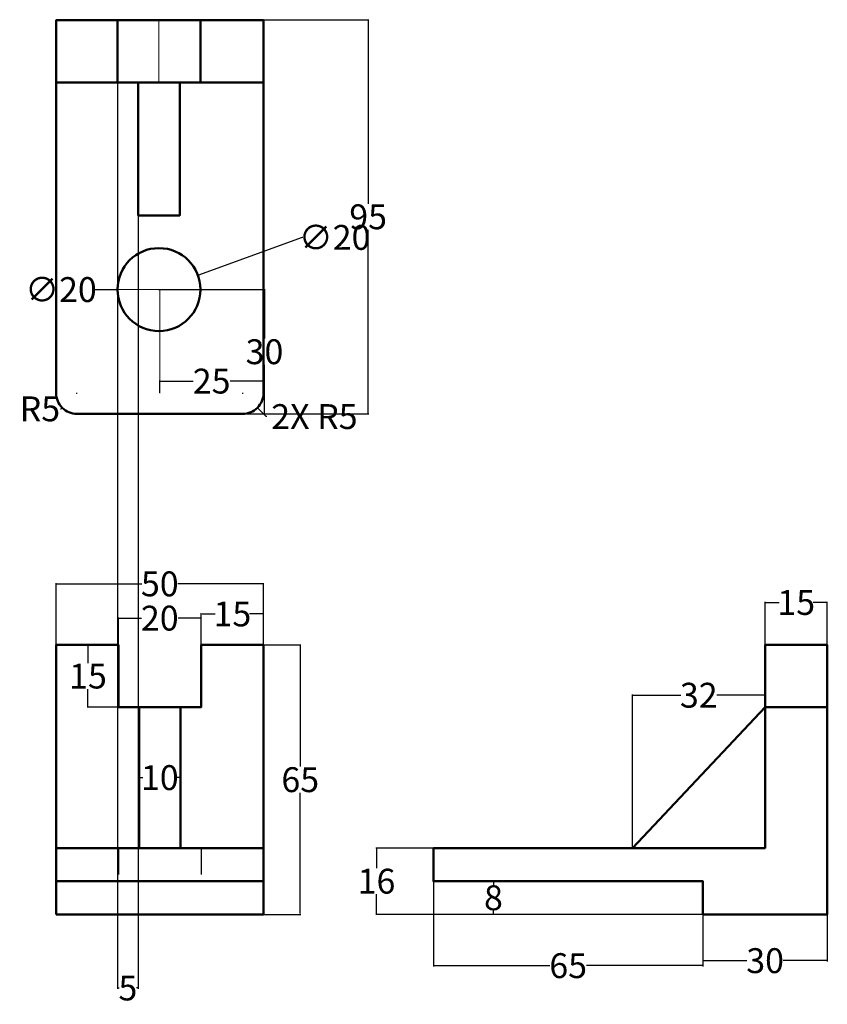
# Model space of a CAD drawing. Units: millimetres. Extents: x 16 to 211, y 7 to 245.
import ezdxf

# ---------------------------------------------------------------- set-up
doc = ezdxf.new("R2010")
doc.units = ezdxf.units.MM
doc.header["$MEASUREMENT"] = 0
doc.linetypes.add('CENTER', pattern=[50.8, 31.75, -6.35, 6.35, -6.35])
doc.linetypes.add('HIDDEN', pattern=[9.525, 6.35, -3.175])
for name, color, linetype, lineweight in [('M-CNTR', 4, 'CENTER', 18), ('M-DIMS', 2, 'Continuous', 25), ('M-HIDN', 3, 'HIDDEN', 25), ('M-OUTL', 7, 'Continuous', 50)]:
    doc.layers.add(name, color=color, linetype=linetype, lineweight=lineweight)
doc.styles.get("Standard").update_dxf_attribs({"font": 'arial.ttf'})
doc.dimstyles.get("Standard").update_dxf_attribs({"dimtxt": 6, "dimasz": 0.18, "dimexe": 0.18, "dimexo": 0.0625, "dimgap": 0.09, "dimtad": 0, "dimtih": 1, "dimtoh": 1, "dimdec": 0, "dimzin": 0, "dimdsep": 46, "dimtxsty": 'Standard', "dimcen": 0.09, "dimadec": 0, "dimazin": 0, "dimtfac": 1, "dimtdec": 0, "dimtofl": 0, "dimtmove": 0, "dimatfit": 3, "dimfxl": 1, "dimtolj": 1, "dimtzin": 0, "dimarcsym": 0})

# ---------------------------------------------------------------- blocks, each defined once
blk = doc.blocks.new('*D1')
at = {"layer": 'Defpoints', "color": 0, "transparency": 16777216}
for p in [(49.66, 245.06), (49.86, 149.94), (100.1, 149.94)]:
    blk.add_point(p, dxfattribs=at)
at = {"layer": 'M-DIMS', "color": 0, "lineweight": -2, "transparency": 16777216}
for p, q in [((49.72, 245.06), (100.28, 245.06)), ((100.1, 244.88), (100.1, 200.66)), ((100.1, 150.12), (100.1, 194.35)), ((49.93, 149.94), (100.28, 149.94))]:
    blk.add_line(p, q, dxfattribs=at)
at = {"layer": 'M-DIMS', "color": 0, "transparency": 16777216}
for points in [[(100.07, 244.88), (100.13, 244.88), (100.1, 245.06)], [(100.07, 150.12), (100.13, 150.12), (100.1, 149.94)]]:
    blk.add_solid(points, dxfattribs=at)
at = {"layer": 'M-DIMS', "color": 0, "transparency": 16777216, "insert": (100.1, 197.5), "char_height": 6, "attachment_point": 5}
blk.add_mtext('\\A1;95', dxfattribs=at)
blk = doc.blocks.new('*D2')
at = {"layer": 'Defpoints', "color": 0, "transparency": 16777216}
for p in [(49.66, 179.94), (49.66, 149.94), (75.1, 149.94)]:
    blk.add_point(p, dxfattribs=at)
at = {"layer": 'M-DIMS', "color": 0, "lineweight": -2, "transparency": 16777216}
for p, q in [((49.72, 179.94), (75.28, 179.94)), ((75.1, 179.76), (75.1, 168.1)), ((75.1, 150.12), (75.1, 161.79)), ((49.72, 149.94), (75.28, 149.94))]:
    blk.add_line(p, q, dxfattribs=at)
at = {"layer": 'M-DIMS', "color": 0, "transparency": 16777216}
for points in [[(75.07, 179.76), (75.13, 179.76), (75.1, 179.94)], [(75.07, 150.12), (75.13, 150.12), (75.1, 149.94)]]:
    blk.add_solid(points, dxfattribs=at)
at = {"layer": 'M-DIMS', "color": 0, "transparency": 16777216, "insert": (75.1, 164.94), "char_height": 6, "attachment_point": 5}
blk.add_mtext('\\A1;30', dxfattribs=at)
blk = doc.blocks.new('*D3')
at = {"layer": 'Defpoints', "color": 0, "transparency": 16777216}
for p in [(59.06, 183.37), (40.27, 176.52)]:
    blk.add_point(p, dxfattribs=at)
at = {"layer": 'M-DIMS', "color": 0, "lineweight": -2, "transparency": 16777216}
for p, q in [((84.2, 192.53), (59.22, 183.43)), ((84.38, 192.53), (84.2, 192.53)), ((49.57, 179.94), (49.75, 179.94)), ((49.66, 179.85), (49.66, 180.03))]:
    blk.add_line(p, q, dxfattribs=at)
at = {"layer": 'M-DIMS', "color": 0, "transparency": 16777216}
blk.add_solid([(59.21, 183.46), (59.23, 183.4), (59.06, 183.37)], dxfattribs=at)
at = {"layer": 'M-DIMS', "color": 0, "transparency": 16777216, "insert": (92.02, 192.53), "char_height": 6, "attachment_point": 5}
blk.add_mtext('\\A1;∅20', dxfattribs=at)
blk = doc.blocks.new('*D4')
at = {"layer": 'Defpoints', "color": 0, "transparency": 16777216}
for p in [(74.86, 157.85), (49.86, 154.94), (74.86, 154.94)]:
    blk.add_point(p, dxfattribs=at)
at = {"layer": 'M-DIMS', "color": 0, "lineweight": -2, "transparency": 16777216}
for p, q in [((49.86, 155.01), (49.86, 158.03)), ((50.04, 157.85), (57.9, 157.85)), ((74.68, 157.85), (66.82, 157.85)), ((74.86, 155.01), (74.86, 158.03))]:
    blk.add_line(p, q, dxfattribs=at)
at = {"layer": 'M-DIMS', "color": 0, "transparency": 16777216}
for points in [[(50.04, 157.88), (50.04, 157.82), (49.86, 157.85)], [(74.68, 157.88), (74.68, 157.82), (74.86, 157.85)]]:
    blk.add_solid(points, dxfattribs=at)
at = {"layer": 'M-DIMS', "color": 0, "transparency": 16777216, "insert": (62.36, 157.85), "char_height": 6, "attachment_point": 5}
blk.add_mtext('\\A1;25', dxfattribs=at)
blk = doc.blocks.new('*D5')
at = {"layer": 'Defpoints', "color": 0, "transparency": 16777216}
for p in [(29.86, 154.94), (26.33, 151.41)]:
    blk.add_point(p, dxfattribs=at)
at = {"layer": 'M-DIMS', "color": 0, "lineweight": -2, "transparency": 16777216}
for p, q in [((29.77, 154.94), (29.95, 154.94)), ((29.86, 154.85), (29.86, 155.03)), ((25.89, 151.15), (26.07, 151.15)), ((26.07, 151.15), (26.2, 151.28))]:
    blk.add_line(p, q, dxfattribs=at)
at = {"layer": 'M-DIMS', "color": 0, "transparency": 16777216}
blk.add_solid([(26.18, 151.3), (26.22, 151.26), (26.33, 151.41)], dxfattribs=at)
at = {"layer": 'M-DIMS', "color": 0, "transparency": 16777216, "insert": (20.94, 151.15), "char_height": 6, "attachment_point": 5}
blk.add_mtext('\\A1;R5', dxfattribs=at)
blk = doc.blocks.new('*D6')
at = {"layer": 'Defpoints', "color": 0, "transparency": 16777216}
for p in [(74.86, 108.92), (24.86, 94.17), (74.86, 94.17)]:
    blk.add_point(p, dxfattribs=at)
at = {"layer": 'M-DIMS', "color": 0, "lineweight": -2, "transparency": 16777216}
for p, q in [((24.86, 94.23), (24.86, 109.1)), ((25.04, 108.92), (45.49, 108.92)), ((74.68, 108.92), (54.24, 108.92)), ((74.86, 94.23), (74.86, 109.1))]:
    blk.add_line(p, q, dxfattribs=at)
at = {"layer": 'M-DIMS', "color": 0, "transparency": 16777216}
for points in [[(25.04, 108.95), (25.04, 108.89), (24.86, 108.92)], [(74.68, 108.95), (74.68, 108.89), (74.86, 108.92)]]:
    blk.add_solid(points, dxfattribs=at)
at = {"layer": 'M-DIMS', "color": 0, "transparency": 16777216, "insert": (49.86, 108.92), "char_height": 6, "attachment_point": 5}
blk.add_mtext('\\A1;50', dxfattribs=at)
blk = doc.blocks.new('*D7')
at = {"layer": 'Defpoints', "color": 0, "transparency": 16777216}
for p in [(39.86, 94.17), (32.54, 79.17), (39.86, 79.17)]:
    blk.add_point(p, dxfattribs=at)
at = {"layer": 'M-DIMS', "color": 0, "lineweight": -2, "transparency": 16777216}
for p, q in [((39.8, 94.17), (32.36, 94.17)), ((32.54, 93.99), (32.54, 89.82)), ((32.54, 79.35), (32.54, 83.52)), ((39.8, 79.17), (32.36, 79.17))]:
    blk.add_line(p, q, dxfattribs=at)
at = {"layer": 'M-DIMS', "color": 0, "transparency": 16777216}
for points in [[(32.51, 93.99), (32.57, 93.99), (32.54, 94.17)], [(32.51, 79.35), (32.57, 79.35), (32.54, 79.17)]]:
    blk.add_solid(points, dxfattribs=at)
at = {"layer": 'M-DIMS', "color": 0, "transparency": 16777216, "insert": (32.54, 86.67), "char_height": 6, "attachment_point": 5}
blk.add_mtext('\\A1;15', dxfattribs=at)
blk = doc.blocks.new('*D8')
at = {"layer": 'Defpoints', "color": 0, "transparency": 16777216}
for p in [(59.86, 100.65), (39.86, 94.17), (59.86, 94.17)]:
    blk.add_point(p, dxfattribs=at)
at = {"layer": 'M-DIMS', "color": 0, "lineweight": -2, "transparency": 16777216}
for p, q in [((39.86, 94.23), (39.86, 100.83)), ((40.04, 100.65), (45.43, 100.65)), ((59.68, 100.65), (54.29, 100.65)), ((59.86, 94.23), (59.86, 100.83))]:
    blk.add_line(p, q, dxfattribs=at)
at = {"layer": 'M-DIMS', "color": 0, "transparency": 16777216}
for points in [[(40.04, 100.68), (40.04, 100.62), (39.86, 100.65)], [(59.68, 100.68), (59.68, 100.62), (59.86, 100.65)]]:
    blk.add_solid(points, dxfattribs=at)
at = {"layer": 'M-DIMS', "color": 0, "transparency": 16777216, "insert": (49.86, 100.65), "char_height": 6, "attachment_point": 5}
blk.add_mtext('\\A1;20', dxfattribs=at)
blk = doc.blocks.new('*D9')
at = {"layer": 'Defpoints', "color": 0, "transparency": 16777216}
for p in [(74.86, 101.66), (59.86, 94.17), (74.86, 94.17)]:
    blk.add_point(p, dxfattribs=at)
at = {"layer": 'M-DIMS', "color": 0, "lineweight": -2, "transparency": 16777216}
for p, q in [((59.86, 94.23), (59.86, 101.84)), ((60.04, 101.66), (63.24, 101.66)), ((74.68, 101.66), (71.49, 101.66)), ((74.86, 94.23), (74.86, 101.84))]:
    blk.add_line(p, q, dxfattribs=at)
at = {"layer": 'M-DIMS', "color": 0, "transparency": 16777216}
for points in [[(60.04, 101.69), (60.04, 101.63), (59.86, 101.66)], [(74.68, 101.69), (74.68, 101.63), (74.86, 101.66)]]:
    blk.add_solid(points, dxfattribs=at)
at = {"layer": 'M-DIMS', "color": 0, "transparency": 16777216, "insert": (67.36, 101.66), "char_height": 6, "attachment_point": 5}
blk.add_mtext('\\A1;15', dxfattribs=at)
blk = doc.blocks.new('*D10')
at = {"layer": 'Defpoints', "color": 0, "transparency": 16777216}
for p in [(44.86, 62.17), (54.86, 62.17), (54.86, 62.17)]:
    blk.add_point(p, dxfattribs=at)
at = {"layer": 'M-DIMS', "color": 0, "lineweight": -2, "transparency": 16777216}
for p, q in [((44.86, 62.23), (44.86, 62.35)), ((45.04, 62.17), (45.77, 62.17)), ((54.68, 62.17), (53.96, 62.17)), ((54.86, 62.23), (54.86, 62.35))]:
    blk.add_line(p, q, dxfattribs=at)
at = {"layer": 'M-DIMS', "color": 0, "transparency": 16777216}
for points in [[(45.04, 62.2), (45.04, 62.14), (44.86, 62.17)], [(54.68, 62.2), (54.68, 62.14), (54.86, 62.17)]]:
    blk.add_solid(points, dxfattribs=at)
at = {"layer": 'M-DIMS', "color": 0, "transparency": 16777216, "insert": (49.86, 62.17), "char_height": 6, "attachment_point": 5}
blk.add_mtext('\\A1;10', dxfattribs=at)
blk = doc.blocks.new('*D11')
at = {"layer": 'Defpoints', "color": 0, "transparency": 16777216}
for p in [(74.86, 94.17), (74.86, 29.17), (83.73, 29.17)]:
    blk.add_point(p, dxfattribs=at)
at = {"layer": 'M-DIMS', "color": 0, "lineweight": -2, "transparency": 16777216}
for p, q in [((74.93, 94.17), (83.91, 94.17)), ((83.73, 93.99), (83.73, 64.82)), ((83.73, 29.35), (83.73, 58.52)), ((74.93, 29.17), (83.91, 29.17))]:
    blk.add_line(p, q, dxfattribs=at)
at = {"layer": 'M-DIMS', "color": 0, "transparency": 16777216}
for points in [[(83.7, 93.99), (83.76, 93.99), (83.73, 94.17)], [(83.7, 29.35), (83.76, 29.35), (83.73, 29.17)]]:
    blk.add_solid(points, dxfattribs=at)
at = {"layer": 'M-DIMS', "color": 0, "transparency": 16777216, "insert": (83.73, 61.67), "char_height": 6, "attachment_point": 5}
blk.add_mtext('\\A1;65', dxfattribs=at)
blk = doc.blocks.new('*D12')
at = {"layer": 'Defpoints', "color": 0, "transparency": 16777216}
for p in [(115.84, 45.17), (102.12, 29.17), (180.84, 29.17)]:
    blk.add_point(p, dxfattribs=at)
at = {"layer": 'M-DIMS', "color": 0, "lineweight": -2, "transparency": 16777216}
for p, q in [((115.77, 45.17), (101.94, 45.17)), ((102.12, 44.99), (102.12, 40.32)), ((102.12, 29.35), (102.12, 34.02)), ((180.77, 29.17), (101.94, 29.17))]:
    blk.add_line(p, q, dxfattribs=at)
at = {"layer": 'M-DIMS', "color": 0, "transparency": 16777216}
for points in [[(102.09, 44.99), (102.15, 44.99), (102.12, 45.17)], [(102.09, 29.35), (102.15, 29.35), (102.12, 29.17)]]:
    blk.add_solid(points, dxfattribs=at)
at = {"layer": 'M-DIMS', "color": 0, "transparency": 16777216, "insert": (102.12, 37.17), "char_height": 6, "attachment_point": 5}
blk.add_mtext('\\A1;16', dxfattribs=at)
blk = doc.blocks.new('*D13')
at = {"layer": 'Defpoints', "color": 0, "transparency": 16777216}
for p in [(180.84, 37.17), (130.32, 29.17), (180.84, 29.17)]:
    blk.add_point(p, dxfattribs=at)
at = {"layer": 'M-DIMS', "color": 0, "lineweight": -2, "transparency": 16777216}
for p, q in [((180.77, 37.17), (130.14, 37.17)), ((130.32, 36.99), (130.32, 36.32)), ((180.77, 29.17), (130.14, 29.17)), ((130.32, 29.35), (130.32, 30.02))]:
    blk.add_line(p, q, dxfattribs=at)
at = {"layer": 'M-DIMS', "color": 0, "transparency": 16777216}
for points in [[(130.29, 36.99), (130.35, 36.99), (130.32, 37.17)], [(130.29, 29.35), (130.35, 29.35), (130.32, 29.17)]]:
    blk.add_solid(points, dxfattribs=at)
at = {"layer": 'M-DIMS', "color": 0, "transparency": 16777216, "insert": (130.32, 33.17), "char_height": 6, "attachment_point": 5}
blk.add_mtext('\\A1;8', dxfattribs=at)
blk = doc.blocks.new('*D14')
at = {"layer": 'Defpoints', "color": 0, "transparency": 16777216}
for p in [(163.84, 82.05), (163.84, 45.17), (195.84, 45.17)]:
    blk.add_point(p, dxfattribs=at)
at = {"layer": 'M-DIMS', "color": 0, "lineweight": -2, "transparency": 16777216}
for p, q in [((163.84, 45.23), (163.84, 82.23)), ((164.02, 82.05), (175.48, 82.05)), ((195.66, 82.05), (184.19, 82.05)), ((195.84, 45.23), (195.84, 82.23))]:
    blk.add_line(p, q, dxfattribs=at)
at = {"layer": 'M-DIMS', "color": 0, "transparency": 16777216}
for points in [[(164.02, 82.08), (164.02, 82.02), (163.84, 82.05)], [(195.66, 82.08), (195.66, 82.02), (195.84, 82.05)]]:
    blk.add_solid(points, dxfattribs=at)
at = {"layer": 'M-DIMS', "color": 0, "transparency": 16777216, "insert": (179.84, 82.05), "char_height": 6, "attachment_point": 5}
blk.add_mtext('\\A1;32', dxfattribs=at)
blk = doc.blocks.new('*D15')
at = {"layer": 'Defpoints', "color": 0, "transparency": 16777216}
for p in [(210.84, 104.43), (195.84, 94.17), (210.84, 94.17)]:
    blk.add_point(p, dxfattribs=at)
at = {"layer": 'M-DIMS', "color": 0, "lineweight": -2, "transparency": 16777216}
for p, q in [((195.84, 94.23), (195.84, 104.61)), ((210.84, 94.23), (210.84, 104.61)), ((196.02, 104.43), (199.21, 104.43)), ((210.66, 104.43), (207.46, 104.43))]:
    blk.add_line(p, q, dxfattribs=at)
at = {"layer": 'M-DIMS', "color": 0, "transparency": 16777216}
for points in [[(196.02, 104.46), (196.02, 104.4), (195.84, 104.43)], [(210.66, 104.46), (210.66, 104.4), (210.84, 104.43)]]:
    blk.add_solid(points, dxfattribs=at)
at = {"layer": 'M-DIMS', "color": 0, "transparency": 16777216, "insert": (203.34, 104.43), "char_height": 6, "attachment_point": 5}
blk.add_mtext('\\A1;15', dxfattribs=at)
blk = doc.blocks.new('*D16')
at = {"layer": 'Defpoints', "color": 0, "transparency": 16777216}
for p in [(115.84, 37.17), (180.84, 37.17), (180.84, 16.79)]:
    blk.add_point(p, dxfattribs=at)
at = {"layer": 'M-DIMS', "color": 0, "lineweight": -2, "transparency": 16777216}
for p, q in [((115.84, 37.11), (115.84, 16.61)), ((180.84, 37.11), (180.84, 16.61)), ((116.02, 16.79), (143.91, 16.79)), ((180.66, 16.79), (152.76, 16.79))]:
    blk.add_line(p, q, dxfattribs=at)
at = {"layer": 'M-DIMS', "color": 0, "transparency": 16777216}
for points in [[(116.02, 16.82), (116.02, 16.76), (115.84, 16.79)], [(180.66, 16.82), (180.66, 16.76), (180.84, 16.79)]]:
    blk.add_solid(points, dxfattribs=at)
at = {"layer": 'M-DIMS', "color": 0, "transparency": 16777216, "insert": (148.34, 16.79), "char_height": 6, "attachment_point": 5}
blk.add_mtext('\\A1;65', dxfattribs=at)
blk = doc.blocks.new('*D17')
at = {"layer": 'Defpoints', "color": 0, "transparency": 16777216}
for p in [(180.84, 29.17), (210.84, 29.17), (210.84, 18)]:
    blk.add_point(p, dxfattribs=at)
at = {"layer": 'M-DIMS', "color": 0, "lineweight": -2, "transparency": 16777216}
for p, q in [((180.84, 29.11), (180.84, 17.82)), ((210.84, 29.11), (210.84, 17.82)), ((181.02, 18), (191.46, 18)), ((210.66, 18), (200.21, 18))]:
    blk.add_line(p, q, dxfattribs=at)
at = {"layer": 'M-DIMS', "color": 0, "transparency": 16777216}
for points in [[(181.02, 18.03), (181.02, 17.97), (180.84, 18)], [(210.66, 18.03), (210.66, 17.97), (210.84, 18)]]:
    blk.add_solid(points, dxfattribs=at)
at = {"layer": 'M-DIMS', "color": 0, "transparency": 16777216, "insert": (195.84, 18), "char_height": 6, "attachment_point": 5}
blk.add_mtext('\\A1;30', dxfattribs=at)
blk = doc.blocks.new('*D18')
at = {"layer": 'Defpoints', "color": 0, "transparency": 16777216}
for p in [(39.66, 229.94), (44.66, 229.82), (44.66, 11.4)]:
    blk.add_point(p, dxfattribs=at)
at = {"layer": 'M-DIMS', "color": 0, "lineweight": -2, "transparency": 16777216}
for p, q in [((39.66, 229.88), (39.66, 11.22)), ((44.66, 229.76), (44.66, 11.22)), ((39.84, 11.4), (40.08, 11.4)), ((44.48, 11.4), (44.24, 11.4))]:
    blk.add_line(p, q, dxfattribs=at)
at = {"layer": 'M-DIMS', "color": 0, "transparency": 16777216}
for points in [[(39.84, 11.43), (39.84, 11.37), (39.66, 11.4)], [(44.48, 11.43), (44.48, 11.37), (44.66, 11.4)]]:
    blk.add_solid(points, dxfattribs=at)
at = {"layer": 'M-DIMS', "color": 0, "transparency": 16777216, "insert": (42.16, 11.4), "char_height": 6, "attachment_point": 5}
blk.add_mtext('\\A1;5', dxfattribs=at)
blk = doc.blocks.new('*D19')
at = {"layer": 'Defpoints', "color": 0, "transparency": 16777216}
for p in [(39.66, 179.94), (59.66, 179.94)]:
    blk.add_point(p, dxfattribs=at)
at = {"layer": 'M-DIMS', "color": 0, "lineweight": -2, "transparency": 16777216}
for p, q in [((33.66, 179.94), (39.48, 179.94)), ((49.57, 179.94), (49.75, 179.94)), ((49.66, 179.85), (49.66, 180.03))]:
    blk.add_line(p, q, dxfattribs=at)
at = {"layer": 'M-DIMS', "color": 0, "transparency": 16777216}
blk.add_solid([(39.48, 179.97), (39.48, 179.91), (39.66, 179.94)], dxfattribs=at)
at = {"layer": 'M-DIMS', "color": 0, "transparency": 16777216, "insert": (26.02, 179.94), "char_height": 6, "attachment_point": 5}
blk.add_mtext('\\A1;∅20', dxfattribs=at)
blk = doc.blocks.new('*D20')
at = {"layer": 'Defpoints', "color": 0, "transparency": 16777216}
for p in [(69.86, 154.94), (73.4, 151.41)]:
    blk.add_point(p, dxfattribs=at)
at = {"layer": 'M-DIMS', "color": 0, "lineweight": -2, "transparency": 16777216}
for p, q in [((69.77, 154.94), (69.95, 154.94)), ((69.86, 154.85), (69.86, 155.03)), ((75.52, 149.29), (73.53, 151.28)), ((75.7, 149.29), (75.52, 149.29))]:
    blk.add_line(p, q, dxfattribs=at)
at = {"layer": 'M-DIMS', "color": 0, "transparency": 16777216}
blk.add_solid([(73.55, 151.3), (73.5, 151.26), (73.4, 151.41)], dxfattribs=at)
at = {"layer": 'M-DIMS', "color": 0, "transparency": 16777216, "insert": (87.15, 149.29), "char_height": 6, "attachment_point": 5}
blk.add_mtext('\\A1;2X R5', dxfattribs=at)

msp = doc.modelspace()

# ---------------------------------------------------------------- linework, layer by layer
at = {"layer": 'M-CNTR'}
for p, q in [((49.66, 229.82), (49.66, 245.06)), ((39.66, 179.94), (59.66, 179.94)), ((49.86, 179.94), (49.86, 154.94)), ((49.86, 29.05), (49.86, 29.17))]:
    msp.add_line(p, q, dxfattribs=at)
at = {"layer": 'M-HIDN'}
for p, q in [((39.86, 45.17), (39.86, 37.17)), ((59.86, 45.17), (59.86, 37.17))]:
    msp.add_line(p, q, dxfattribs=at)
at = {"layer": 'M-OUTL'}
for p, q in [((39.66, 229.94), (39.66, 244.94)), ((59.66, 229.94), (59.66, 244.94)), ((24.86, 229.94), (74.86, 229.94)), ((54.86, 45.17), (54.86, 79.17)), ((24.86, 45.17), (74.86, 45.17)), ((24.86, 37.17), (74.86, 37.17))]:
    msp.add_line(p, q, dxfattribs=at)
msp.add_lwpolyline([(24.86, 154.94, 0.414214), (29.86, 149.94), (69.86, 149.94, 0.414214), (74.86, 154.94), (74.86, 244.94), (24.86, 244.94)], format="xyb", close=True, dxfattribs=at)
for points in [[(44.66, 229.82), (44.66, 197.82), (54.66, 197.82), (54.66, 229.82)], [(210.84, 79.17), (195.84, 79.17), (163.84, 45.17)]]:
    msp.add_lwpolyline(points, dxfattribs=at)
for points in [[(24.86, 29.17), (24.86, 94.17), (39.86, 94.17), (39.86, 79.17), (59.86, 79.17), (59.86, 94.17), (74.86, 94.17), (74.86, 29.17)], [(115.84, 45.17), (115.84, 37.17), (180.84, 37.17), (180.84, 29.17), (210.84, 29.17), (210.84, 94.17), (195.84, 94.17), (195.84, 45.17), (190.84, 45.17)], [(44.86, 45.17), (44.86, 79.17)]]:
    msp.add_lwpolyline(points, close=True, dxfattribs=at)
msp.add_circle((49.66, 179.94), 10, dxfattribs=at)

# ---------------------------------------------------------------- dimensions: what is measured, and where the dimension line sits
at = {"layer": 'M-DIMS'}
for base, p1, p2, picture, middle in [((100.1, 149.94), (49.66, 245.06), (49.86, 149.94), '*D1', (100.1, 197.5)), ((75.1, 149.94), (49.66, 179.94), (49.66, 149.94), '*D2', (75.1, 164.94)), ((32.54, 79.17), (39.86, 94.17), (39.86, 79.17), '*D7', (32.54, 86.67)), ((83.73, 29.17), (74.86, 94.17), (74.86, 29.17), '*D11', (83.73, 61.67)), ((102.12, 29.17), (115.84, 45.17), (180.84, 29.17), '*D12', (102.12, 37.17)), ((130.32, 29.17), (180.84, 37.17), (180.84, 29.17), '*D13', (130.32, 33.17))]:
    dim = msp.add_linear_dim(base=base, p1=p1, p2=p2, angle=90, dimstyle='Standard', override={"dimclrd": 0, "dimclre": 0, "dimclrt": 0}, dxfattribs=at)
    dim.commit()
    dim.dimension.update_dxf_attribs({"geometry": picture, "text_midpoint": middle})
for base, p1, p2, override, picture, middle in [((44.66, 11.4), (39.66, 229.94), (44.66, 229.82), {"dimdec": 0, "dimlfac": 1, "dimrnd": 0, "dimzin": 0, "dimdsep": 46, "dimlunit": 2}, '*D18', (42.16, 11.4)), ((74.86, 157.85), (49.86, 154.94), (74.86, 154.94), {"dimclrd": 0, "dimclre": 0, "dimclrt": 0}, '*D4', (62.36, 157.85)), ((74.86, 108.92), (24.86, 94.17), (74.86, 94.17), {"dimclrd": 0, "dimclre": 0, "dimclrt": 0}, '*D6', (49.86, 108.92)), ((210.84, 104.43), (195.84, 94.17), (210.84, 94.17), {"dimclrd": 0, "dimclre": 0, "dimclrt": 0}, '*D15', (203.34, 104.43)), ((59.86, 100.65), (39.86, 94.17), (59.86, 94.17), {"dimclrd": 0, "dimclre": 0, "dimclrt": 0}, '*D8', (49.86, 100.65)), ((74.86, 101.66), (59.86, 94.17), (74.86, 94.17), {"dimclrd": 0, "dimclre": 0, "dimclrt": 0}, '*D9', (67.36, 101.66)), ((163.84, 82.05), (195.84, 45.17), (163.84, 45.17), {"dimclrd": 0, "dimclre": 0, "dimclrt": 0}, '*D14', (179.84, 82.05)), ((54.86, 62.17), (44.86, 62.17), (54.86, 62.17), {"dimclrd": 0, "dimclre": 0, "dimclrt": 0}, '*D10', (49.86, 62.17)), ((180.84, 16.79), (115.84, 37.17), (180.84, 37.17), {"dimclrd": 0, "dimclre": 0, "dimclrt": 0}, '*D16', (148.34, 16.79)), ((210.84, 18), (180.84, 29.17), (210.84, 29.17), {"dimclrd": 0, "dimclre": 0, "dimclrt": 0}, '*D17', (195.84, 18))]:
    dim = msp.add_linear_dim(base=base, p1=p1, p2=p2, dimstyle='Standard', override=override, dxfattribs=at)
    dim.commit()
    dim.dimension.update_dxf_attribs({"geometry": picture, "text_midpoint": middle})
for p1, p2, override, picture, middle in [((40.27, 176.52), (59.06, 183.37), {"dimclrd": 0, "dimclre": 0, "dimclrt": 0}, '*D3', (92.02, 192.53)), ((59.66, 179.94), (39.66, 179.94), {"dimdec": 0, "dimlfac": 1, "dimrnd": 0, "dimzin": 0, "dimdsep": 46, "dimlunit": 2}, '*D19', (33.66, 179.94))]:
    dim = msp.add_diameter_dim_2p(p1=p1, p2=p2, dimstyle='Standard', override=override, dxfattribs=at)
    dim.commit()
    dim.dimension.update_dxf_attribs({"geometry": picture, "text_midpoint": middle, "dimtype": 163})
dim = msp.add_radius_dim(center=(69.86, 154.94), mpoint=(73.4, 151.41), text='2X <>', dimstyle='Standard', override={"dimdec": 0, "dimlfac": 1, "dimrnd": 0, "dimzin": 0, "dimdsep": 46, "dimlunit": 2}, dxfattribs=at)
dim.commit()
dim.dimension.update_dxf_attribs({"geometry": '*D20', "text_midpoint": (87.15, 149.29), "dimtype": 164})
dim = msp.add_radius_dim(center=(29.86, 154.94), mpoint=(26.33, 151.41), dimstyle='Standard', override={"dimclrd": 0, "dimclre": 0, "dimclrt": 0}, dxfattribs=at)
dim.commit()
dim.dimension.update_dxf_attribs({"geometry": '*D5', "text_midpoint": (20.94, 151.15)})

doc.saveas('drawing.dxf')
